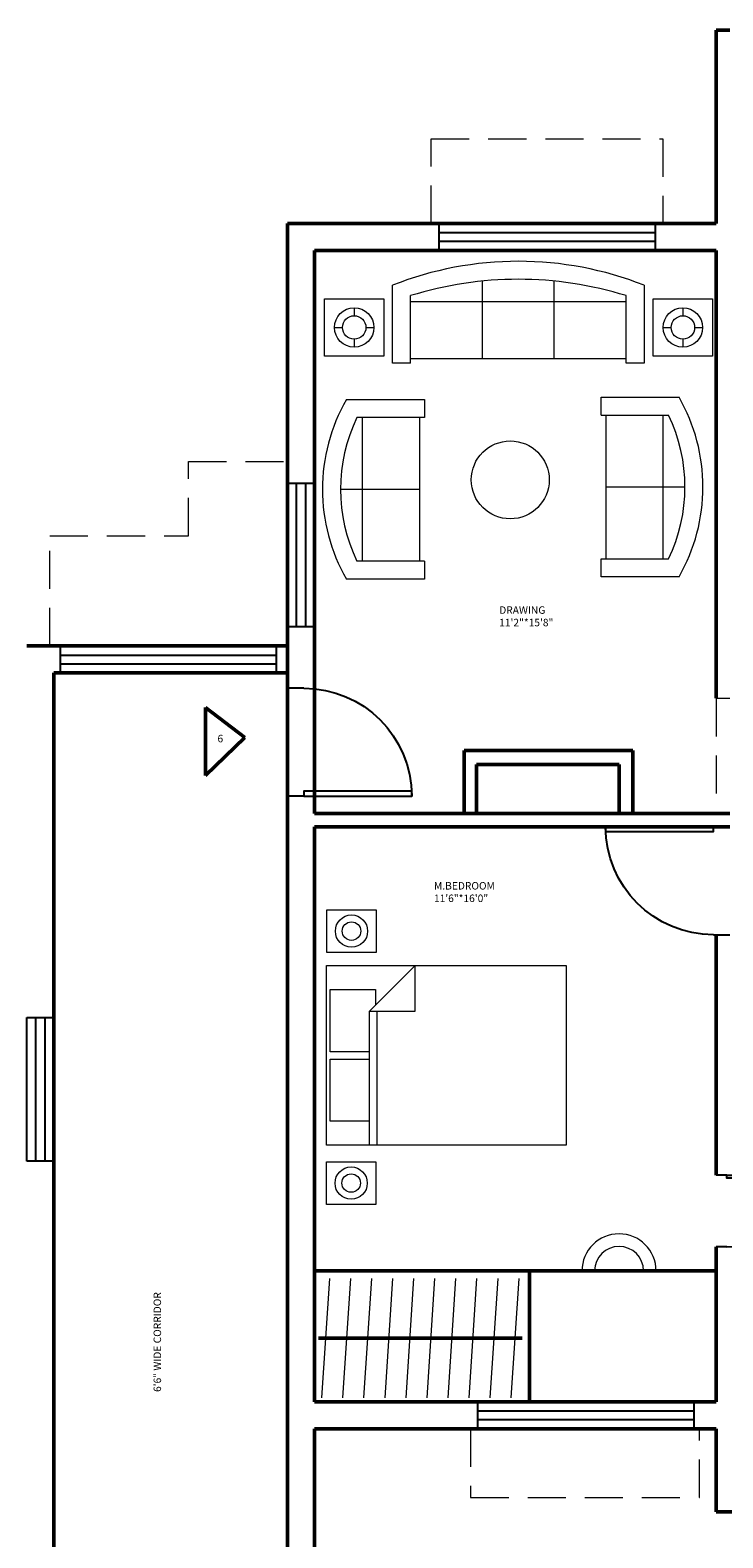
# Model space of a CAD drawing. Units: inches. Extents: x 291 to 2631, y 456 to 2623.
# Tile 20 of 22: x 1974 to 2205, y 2120 to 2623. Entities that reach past the tile are written whole.
import ezdxf

# ---------------------------------------------------------------- set-up
doc = ezdxf.new("R2010")
doc.units = ezdxf.units.IN
doc.linetypes.add('DASHED', pattern=[19.05, 12.7, -6.35])
for name, color, linetype, lineweight in [('A-ANNO-TEXT', 3, 'Continuous', 25), ('A-AREA-IDEN', 7, 'Continuous', 25), ('A-DOOR', 3, 'Continuous', 25), ('A-FLOR-OVHD', 1, 'DASHED', 18), ('A-FURN', 8, 'Continuous', 18), ('A-GLAZ', 4, 'Continuous', 25), ('A-WALL', 7, 'Continuous', 50)]:
    doc.layers.add(name, color=color, linetype=linetype, lineweight=lineweight)
doc.styles.get("Standard").update_dxf_attribs({"font": 'arial.ttf'})

# ---------------------------------------------------------------- blocks, each defined once
blk = doc.blocks.new('*U2')
for p, q in [((0, 0), (0, -6)), ((40, 0), (40, -6))]:
    blk.add_line(p, q)
blk.add_lwpolyline([(0, 0), (0, 40), (1.75, 40), (1.75, 0)], close=True)
blk.add_arc((0, 0), 40, 0, 90)
blk = doc.blocks.new('Sofa - Roundback 7 ft.')
for p, q in [((-12.00002, -32.4421), (-12.00003, -6.5971)), ((11.99997, -32.4421), (11.99998, -6.5971)), ((-36.000027, -34), (-36.000027, -11.4696)), ((-35.999844, -13.3819), (35.9998, -13.3819)), ((35.99998, -34), (35.99998, -11.4696)), ((-36.000027, -32.4421), (35.99998, -32.4421))]:
    blk.add_line(p, q)
for points in [[(-36.000027, -34), (-42.000027, -34), (-42.000027, -8)], [(41.99998, -8), (41.99998, -34), (35.99998, -34)]]:
    blk.add_lwpolyline(points)
for centre, radius, start, end in [((0, -114.25), 114.25, 68.43141, 111.5686), ((-0.00001, -127.1968), 121.1968, 72.72033, 107.2797)]:
    blk.add_arc(centre, radius, start, end)
blk = doc.blocks.new('Sofa - Roundback Loveseat 5 ft.')
for p, q in [((0, -32.44198), (0, -5.99998)), ((-24, -33.99998), (-24, -11.46958)), ((-23.9998, -13.38178), (23.99986, -13.38178)), ((24.00004, -33.99998), (24.00004, -11.46958)), ((-24, -32.44198), (24.00004, -32.44198))]:
    blk.add_line(p, q)
for points in [[(-24, -33.99998), (-30, -33.99998), (-30, -7.99998)], [(30.00004, -7.99998), (30.00004, -33.99998), (24.00004, -33.99998)]]:
    blk.add_lwpolyline(points)
for centre, radius, start, end in [((0, -60.24998), 60.24998, 60.13715, 119.8628), ((0, -61.38438), 55.38444, 64.32083, 115.6792)]:
    blk.add_arc(centre, radius, start, end)
blk = doc.blocks.new('Bed - Queen')
for p, q in [((0, -80.00003), (0, 0)), ((0, 0), (59.99999, 0)), ((59.99999, 0), (59.99999, -80.00003)), ((7.99999, -1.2), (28.79998, -1.2)), ((7.99999, -14.4), (7.99999, -1.2)), ((28.79998, -1.2), (28.79998, -14.4)), ((31.19999, -1.2), (51.99999, -1.2)), ((31.19999, -14.4), (31.19999, -1.2)), ((51.99999, -1.2), (51.99999, -16.4)), ((0, -14.4), (44.8, -14.4)), ((59.99999, -29.6), (44.8, -14.4)), ((44.8, -14.4), (44.8, -29.6)), ((44.8, -16.8), (0, -16.8)), ((51.99999, -16.4), (46.79936, -16.4)), ((44.8, -29.6), (59.99999, -29.6)), ((59.99999, -80.00003), (0, -80.00003))]:
    blk.add_line(p, q)
blk = doc.blocks.new('WIN-1800')
for p, q in [((0, 9), (72, 9)), ((0, 0), (0, 9)), ((0, 6), (72, 6)), ((72, 9), (72, 0)), ((72, 3), (0, 3)), ((72, 0), (0, 0))]:
    blk.add_line(p, q)
blk = doc.blocks.new('WIN-1200')
for p, q in [((0, 0), (0, 48)), ((0, 48), (9, 48)), ((3, 0), (3, 48)), ((6, 48), (6, 0)), ((9, 48), (9, 0)), ((9, 0), (0, 0))]:
    blk.add_line(p, q)
blk = doc.blocks.new('LAMP-C')
for p, q in [((9.9, 16.15), (9.9, 13.47)), ((3.32, 9.57), (5.99, 9.57)), ((9.9, 5.66), (9.9, 2.99)), ((13.8, 9.57), (16.48, 9.57))]:
    blk.add_line(p, q)
blk.add_lwpolyline([(0, 19.13), (19.79, 19.13), (19.79, 0), (0, 0)], close=True)
for radius in [6.58, 3.91]:
    blk.add_circle((9.9, 9.57), radius)

msp = doc.modelspace()

# ---------------------------------------------------------------- linework, layer by layer
at = {"layer": 'A-FLOR-OVHD'}
for p, q in [((2107.4, 2558.74), (2107.4, 2587.02)), ((2107.4, 2587.02), (2184.7, 2587.02)), ((2184.7, 2587.02), (2184.7, 2558.74)), ((2026.38, 2454.45), (2026.38, 2479.3)), ((2026.38, 2479.3), (2059.49, 2479.3)), ((1980.17, 2417.68), (1980.17, 2454.45)), ((1980.17, 2454.45), (2026.38, 2454.45)), ((2202.49, 2400.18), (2206.99, 2400.18)), ((2202.49, 2400.18), (2202.49, 2361.74)), ((2120.56, 2156.24), (2120.56, 2133.35)), ((2196.95, 2133.35), (2196.95, 2156.24)), ((2120.56, 2133.35), (2196.95, 2133.35))]:
    msp.add_line(p, q, dxfattribs=at)
at = {"layer": 'A-FURN'}
for p, q in [((2070.95, 2166.64), (2073.6, 2206.52)), ((2077.96, 2166.64), (2080.61, 2206.52)), ((2084.97, 2166.64), (2087.62, 2206.52)), ((2091.99, 2166.64), (2094.63, 2206.52)), ((2099, 2166.64), (2101.65, 2206.52)), ((2106.01, 2166.64), (2108.66, 2206.52)), ((2113.02, 2166.64), (2115.67, 2206.52)), ((2120.04, 2166.64), (2122.68, 2206.52)), ((2127.05, 2166.64), (2129.7, 2206.52)), ((2134.06, 2166.64), (2136.71, 2206.52))]:
    msp.add_line(p, q, dxfattribs=at)
for points in [[(2072.57, 2329.6), (2089.05, 2329.6), (2089.05, 2315.3), (2072.57, 2315.3)], [(2072.46, 2245.47), (2088.94, 2245.47), (2088.94, 2231.17), (2072.46, 2231.17)]]:
    msp.add_lwpolyline(points, close=True, dxfattribs=at)
for centre, radius in [((2133.78, 2473.12), 13), ((2080.81, 2322.45), 5.39), ((2080.81, 2322.45), 3.08), ((2080.7, 2238.32), 5.39), ((2080.7, 2238.32), 3.08)]:
    msp.add_circle(centre, radius, dxfattribs=at)
for radius in [12.37, 8.17]:
    msp.add_arc((2170.07, 2209.01), radius, 0, 180, dxfattribs=at)
at = {"layer": 'A-WALL'}
for p, q in [((2202.49, 2558.74), (2202.49, 2623.27)), ((2202.49, 2623.27), (2206.99, 2623.27)), ((2059.49, 2558.74), (2059.49, 2156.24)), ((2059.49, 2558.74), (2202.49, 2558.74)), ((2068.49, 2549.74), (2068.49, 2361.74)), ((2068.49, 2549.74), (2202.49, 2549.74)), ((2202.49, 2549.74), (2202.49, 2400.18)), ((2059.49, 2417.68), (1972.49, 2417.68)), ((2059.49, 2408.68), (1981.49, 2408.68)), ((1981.49, 2408.68), (1981.49, 2156.24)), ((2032.1, 2397.13), (2032.1, 2374.41)), ((2045.2, 2387.13), (2032.1, 2397.13)), ((2032.1, 2374.41), (2045.2, 2387.13)), ((2118.39, 2361.74), (2118.39, 2382.71)), ((2118.39, 2382.71), (2174.68, 2382.71)), ((2174.68, 2382.71), (2174.68, 2361.74)), ((2122.55, 2361.74), (2122.55, 2378.08)), ((2122.55, 2378.08), (2170.07, 2378.08)), ((2170.07, 2378.08), (2170.07, 2361.74)), ((2068.49, 2361.74), (2206.99, 2361.74)), ((2068.49, 2357.24), (2206.99, 2357.24)), ((2068.49, 2357.24), (2068.49, 2165.24)), ((2202.49, 2321.24), (2202.49, 2241)), ((2202.49, 2217), (2202.49, 2165.24)), ((2068.49, 2209.01), (2202.49, 2209.01)), ((2140.18, 2209.01), (2140.18, 2165.24)), ((2069.83, 2186.58), (2137.7, 2186.58)), ((2068.49, 2165.24), (2202.49, 2165.24)), ((1981.49, 2156.24), (1981.49, 1804.93)), ((2059.49, 2156.24), (2059.49, 1916.04)), ((2068.49, 2156.24), (2202.49, 2156.24)), ((2068.49, 2156.24), (2068.49, 1916.12)), ((2202.49, 2156.24), (2202.49, 2128.54)), ((2202.49, 2128.54), (2271.49, 2128.54))]:
    msp.add_line(p, q, dxfattribs=at)

# ---------------------------------------------------------------- block references
at = {"layer": 'A-DOOR'}
for p, xscale, yscale, zscale, rotation in [((2064.89, 2367.55), -0.9, 0.9, 0.9, 270), ((2201.59, 2357.24), -0.9, 0.9, 0.9, 90), ((2206.09, 2241), 0.6, 0.6, 0.6, 270)]:
    msp.add_blockref('*U2', p, dxfattribs=dict(at, xscale=xscale, yscale=yscale, zscale=zscale, rotation=rotation))
at = {"layer": 'A-FURN'}
for name, p in [('Sofa - Roundback 7 ft.', (2136.48, 2546.09)), ('LAMP-C', (2071.81, 2514.43)), ('LAMP-C', (2181.48, 2514.43))]:
    msp.add_blockref(name, p, dxfattribs=at)
for name, p, rotation in [('Sofa - Roundback Loveseat 5 ft.', (2071.13, 2469.95), 90), ('Sofa - Roundback Loveseat 5 ft.', (2198.08, 2470.74), 270.0000000000006), ('Bed - Queen', (2072.46, 2250.95), 90)]:
    msp.add_blockref(name, p, dxfattribs=dict(at, rotation=rotation))
at = {"layer": 'A-GLAZ'}
for name, p in [('WIN-1800', (2110.09, 2549.74)), ('WIN-1200', (2059.49, 2424.03)), ('WIN-1800', (1983.71, 2408.61)), ('WIN-1200', (1972.49, 2245.61)), ('WIN-1800', (2123, 2156.24))]:
    msp.add_blockref(name, p, dxfattribs=at)

# ---------------------------------------------------------------- texts
at = {"layer": 'A-ANNO-TEXT', "insert": (2036.11, 2387.99), "char_height": 2.5, "attachment_point": 1}
msp.add_mtext_dynamic_manual_height_columns('6', width=6.3236, gutter_width=12.5, heights=[0], dxfattribs=at)
at = {"layer": 'A-AREA-IDEN', "char_height": 2.5, "attachment_point": 1}
for s, width, insert in [('DRAWING\\P11\'2"*15\'8"', 74.8986, (2130.09, 2430.89)), ('M.BEDROOM\\P11\'6"*16\'0"', 55.5416, (2108.33, 2338.83))]:
    msp.add_mtext_dynamic_manual_height_columns(s, width=width, gutter_width=12.5, heights=[0], dxfattribs=dict(at, insert=insert))
at = {"layer": 'A-AREA-IDEN', "insert": (2014.78, 2168.59), "char_height": 2.5, "attachment_point": 1, "rotation": 90}
msp.add_mtext_dynamic_manual_height_columns('6\'6" WIDE CORRIDOR', width=61.1173, gutter_width=12.5, heights=[0], dxfattribs=at)

doc.saveas('drawing.dxf')
